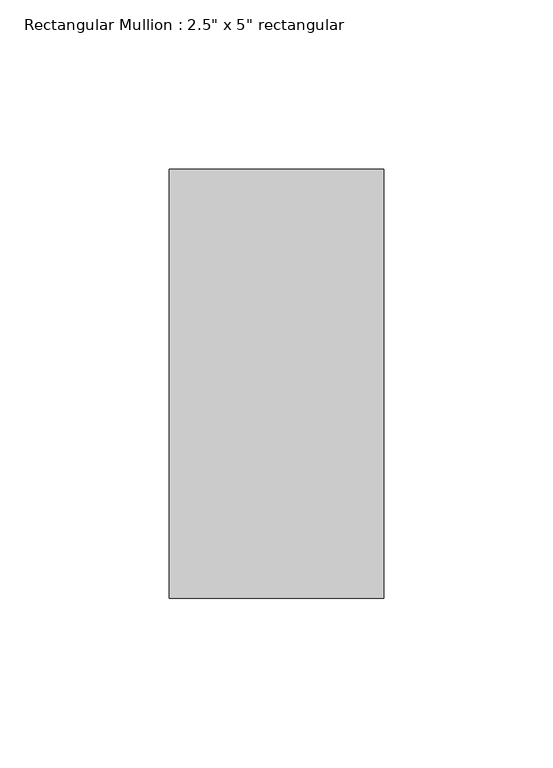
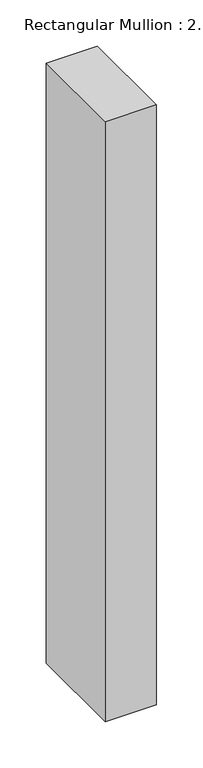
"""IFC4 building model written with IfcOpenShell, lengths in millimetres: member geometry."""

from ifc_helpers import new_model, si_unit, frame, origin, place, context, project, spatial, polyline, outline, extrude, source, transform, mapped, element, save


def member_90be0342(model_context):
    return source(origin(), model_context, "Body", "SweptSolid", [
        extrude(outline(polyline([(31.75, 63.5), (31.75, -63.5), (-31.75, -63.5), (-31.75, 63.5), (31.75, 63.5)])), frame((0.0, 0.0, -788.6592248), z_axis=(0.0, 0.0, 1.0), x_axis=(1.0, 0.0, 0.0)), (0.0, 0.0, 1.0), 788.6592248),
    ])


if __name__ == "__main__":
    model = new_model("IFC4")
    model_context = context("Model", 3, world=origin())
    ifc_project = project(units=[si_unit("LENGTHUNIT", "METRE", prefix="MILLI")], contexts=[model_context])
    site = spatial("IfcSite", under=ifc_project)
    building = spatial("IfcBuilding", under=site)
    placement = place(None, origin())
    member_shape = member_90be0342(model_context)
    element("IfcMember", 1, ObjectType="Rectangular Mullion : 2.5\" x 5\" rectangular", at=placement, inside=building, context=model_context, shape_type="MappedRepresentation", body=[
        mapped(member_shape, transform((0.0, 0.0, 0.0), x_axis=(1.0, 0.0, 0.0), y_axis=(0.0, 1.0, 0.0), z_axis=(0.0, 0.0, 1.0))),
    ])
    save(model, "model.ifc")

# Revit data of these elements
# Type "Rectangular Mullion : 2.5\" x 5\" rectangular"
#   built-in parameter 1007304 = 0.416667 (stored number, unit not read)
#   built-in parameter 1007301 = 0.104167 (stored number, unit not read)
#   built-in parameter 1007300 = 0.104167 (stored number, unit not read)
# Element 1 (IfcMember, "Rectangular Mullion : 2.5\" x 5\" rectangular")
#   Materials on its faces: "Roofing, EPDM Membrane"
# Materials
#   "Roofing, EPDM Membrane": class "Generic", colour RGB 127 127 127, transparency 0, Description = "EPDM roof membrane", Cost = 0
